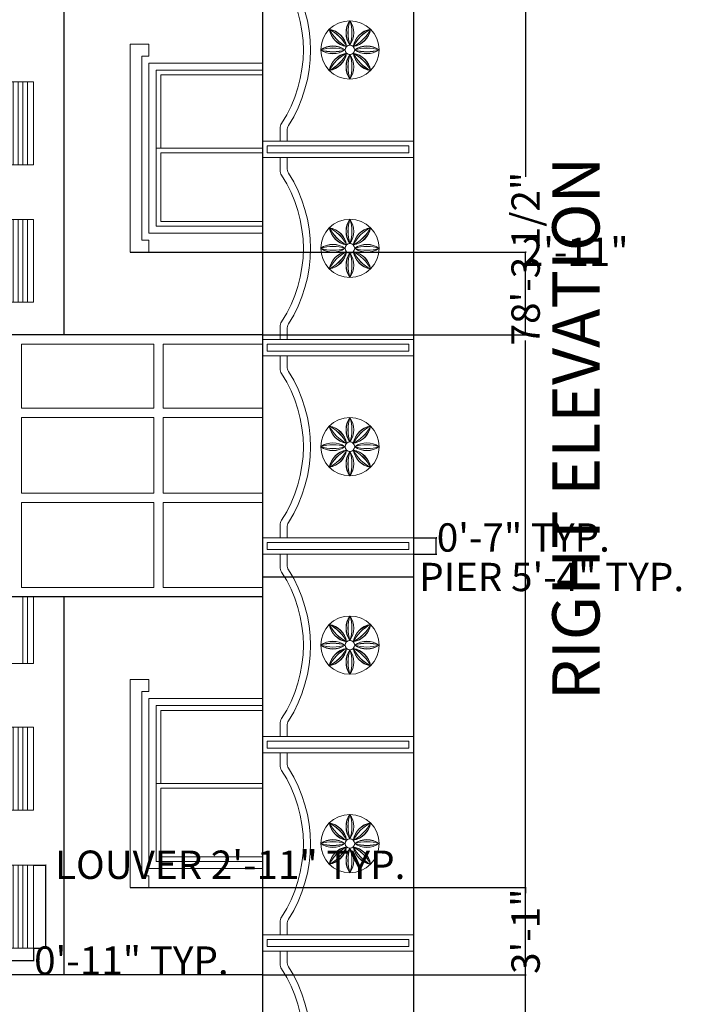
# Model space of a CAD drawing. Units: inches. Extents: x 1146 to 2917, y 889 to 2437.
# Tile 12 of 13: x 2585 to 2865, y 1586 to 2003. Entities that reach past the tile are written whole.
import ezdxf

# ---------------------------------------------------------------- set-up
doc = ezdxf.new("R2010")
doc.units = ezdxf.units.IN
doc.header["$MEASUREMENT"] = 0
for name, color, linetype, lineweight in [('A-ANNO-DIMS', 2, 'Continuous', 18), ('A-ANNO-TEXT', 7, 'Continuous', 25), ('A-ELEV', 7, 'Continuous', 30), ('A-ELEV-GLAZ', 5, 'Continuous', 18), ('A-ELEV-ORNM', 8, 'Continuous', 18)]:
    doc.layers.add(name, color=color, linetype=linetype, lineweight=lineweight)
doc.styles.get("Standard").update_dxf_attribs({"font": 'arial.ttf'})
doc.dimstyles.get("Standard").update_dxf_attribs({"dimtxt": 12, "dimasz": 0.18, "dimexe": 0.18, "dimexo": 0.0625, "dimgap": 0.09, "dimtad": 0, "dimtoh": 1, "dimdec": 1, "dimzin": 0, "dimdsep": 46, "dimlunit": 4, "dimtxsty": 'Standard', "dimcen": 0.09, "dimadec": 0, "dimazin": 0, "dimtfac": 1, "dimtdec": 1, "dimtofl": 0, "dimtmove": 0, "dimatfit": 3, "dimfxl": 1, "dimtolj": 1, "dimtzin": 0, "dimarcsym": 0})

# ---------------------------------------------------------------- blocks, each defined once
blk = doc.blocks.new('BOUNDARY-WALL-PIER')
for points in [[(0, 6.94), (64, 6.94), (64, 0), (0, 0)], [(2, 4.94), (62, 4.94), (62, 2), (2, 2)]]:
    blk.add_lwpolyline(points, close=True)
blk = doc.blocks.new('PARAPET-LOUVER')
for p, q in [((2.58, 0), (2.58, 35.13)), ((4.58, 0), (4.58, 35.13)), ((6.58, 0), (6.58, 35.13)), ((8.58, 0), (8.58, 35.13))]:
    blk.add_line(p, q)
blk.add_lwpolyline([(0, 0), (11.07, 0), (11.07, 35.13), (0, 35.13)], close=True)
blk = doc.blocks.new('WINDOW-ELEV-72')
for p, q in [((8, 83), (8, 88)), ((11, 44), (11, 77)), ((11, 77), (56, 77)), ((11, 11), (11, 44)), ((56, 44), (11, 44)), ((56, 11), (11, 11)), ((7.96, 5), (7.96, 0))]:
    blk.add_line(p, q)
for points in [[(7.96, 0), (0, 0), (0, 88), (8, 88)], [(7.96, 5), (5, 5), (5, 83), (8, 83)], [(56, 8), (8, 8), (8, 80), (56, 80)], [(13, 44), (13, 75), (56, 75)], [(13, 42), (56, 42)], [(56, 13), (13, 13), (13, 42)]]:
    blk.add_lwpolyline(points)
blk = doc.blocks.new('BOUNDARY-WALL-ARCH-CAP')
for p, q in [((0, 71.74), (0, 77.06)), ((3, 72.62), (3, 77.06)), ((0, 0), (0, 5.32)), ((3, 0), (3, 4.44))]:
    blk.add_line(p, q)
for centre, radius, start, end in [((4, 71.74), 4, 180, 213.079), ((7, 72.62), 4, 180, 212.2708), ((-46.98, 38.53), 56.85, 326.921, 33.079), ((-46.98, 38.53), 59.85, 327.7292, 32.2708), ((4, 5.32), 4, 146.921, 180), ((7, 4.44), 4, 147.7292, 180)]:
    blk.add_arc(centre, radius, start, end)
blk = doc.blocks.new('ROSETTE-PLANAR-TRACERY')
for radius in [12.33, 2.02]:
    blk.add_circle((12.33, 12.33), radius)
for centre, radius, start, end in [((2.21, 12.37), 8.8, 9.1552, 80.8448), ((12.65, 22.8), 9.21, 190.95, 259.05), ((19.96, 19.51), 9.21, 145.95, 214.05), ((5.2, 19.51), 8.8, 324.1552, 35.8448), ((12.37, 22.46), 8.8, 279.1552, 350.8448), ((22.8, 12.02), 9.21, 100.95, 169.05), ((5.15, 5.2), 8.8, 54.1552, 125.8448), ((19.51, 4.71), 9.21, 55.95, 124.05), ((5.15, 19.96), 9.21, 235.95, 304.05), ((12.3, 2.21), 8.8, 99.1552, 170.8448), ((1.86, 12.65), 9.21, 280.95, 349.05), ((19.47, 5.15), 8.8, 144.1552, 215.8448), ((4.71, 5.15), 9.21, 325.95, 34.05), ((22.46, 12.3), 8.8, 189.1552, 260.8448), ((12.02, 1.86), 9.21, 10.95, 79.05), ((19.51, 19.47), 8.8, 234.1552, 305.8448)]:
    blk.add_arc(centre, radius, start, end)
at = {"extrusion": (-2e-16, -2e-16, -1)}
for centre, radius, start, end in [((-12.3, 22.46), 8.8, 279.1552, 350.8448), ((-1.86, 12.02), 9.21, 100.95, 169.05)]:
    blk.add_arc(centre, radius, start, end, dxfattribs=at)
at = {"extrusion": (-2e-16, 0, -1)}
for centre, radius, start, end in [((-19.47, 19.51), 8.8, 324.1552, 35.8448), ((-4.71, 19.51), 9.21, 145.95, 214.05)]:
    blk.add_arc(centre, radius, start, end, dxfattribs=at)
at = {"extrusion": (-2e-16, 2e-16, -1)}
for centre, radius, start, end in [((-22.46, 12.37), 8.8, 9.1552, 80.8448), ((-12.02, 22.8), 9.21, 190.95, 259.05)]:
    blk.add_arc(centre, radius, start, end, dxfattribs=at)
at = {"extrusion": (0, -2e-16, -1)}
for centre, radius, start, end in [((-5.15, 4.71), 9.21, 55.95, 124.05), ((-5.15, 19.47), 8.8, 234.1552, 305.8448)]:
    blk.add_arc(centre, radius, start, end, dxfattribs=at)
at = {"extrusion": (0, 2e-16, -1)}
for centre, radius, start, end in [((-19.51, 5.2), 8.8, 54.1552, 125.8448), ((-19.51, 19.96), 9.21, 235.95, 304.05)]:
    blk.add_arc(centre, radius, start, end, dxfattribs=at)
at = {"extrusion": (2e-16, -2e-16, -1)}
for centre, radius, start, end in [((-2.21, 12.3), 8.8, 189.1552, 260.8448), ((-12.65, 1.86), 9.21, 10.95, 79.05)]:
    blk.add_arc(centre, radius, start, end, dxfattribs=at)
at = {"extrusion": (2e-16, 0, -1)}
for centre, radius, start, end in [((-19.96, 5.15), 9.21, 325.95, 34.05), ((-5.2, 5.15), 8.8, 144.1552, 215.8448)]:
    blk.add_arc(centre, radius, start, end, dxfattribs=at)
at = {"extrusion": (2e-16, 2e-16, -1)}
for centre, radius, start, end in [((-12.37, 2.21), 8.8, 99.1552, 170.8448), ((-22.8, 12.65), 9.21, 280.95, 349.05)]:
    blk.add_arc(centre, radius, start, end, dxfattribs=at)
blk = doc.blocks.new('*D83')
at = {"layer": 'A-ANNO-DIMS', "color": 0, "lineweight": -2, "transparency": 16777216}
for p, q in [((2688.2, 1776.39), (2688.2, 1766.67)), ((2752.2, 1776.39), (2752.2, 1766.67)), ((2688.38, 1766.85), (2752.02, 1766.85)), ((2752.2, 1766.85), (2752.38, 1766.85))]:
    blk.add_line(p, q, dxfattribs=at)
at = {"layer": 'A-ANNO-DIMS', "color": 0, "transparency": 16777216}
for points in [[(2688.38, 1766.88), (2688.38, 1766.82), (2688.2, 1766.85)], [(2752.02, 1766.88), (2752.02, 1766.82), (2752.2, 1766.85)]]:
    blk.add_solid(points, dxfattribs=at)
at = {"layer": 'Defpoints', "color": 0, "transparency": 16777216}
for p in [(2688.2, 1776.45), (2752.2, 1776.45), (2752.2, 1766.85)]:
    blk.add_point(p, dxfattribs=at)
at = {"layer": 'A-ANNO-DIMS', "color": 0, "transparency": 16777216, "insert": (2810.64, 1766.85), "char_height": 12, "attachment_point": 5}
blk.add_mtext('\\A1;PIER 5\'-4" TYP.', dxfattribs=at)
blk = doc.blocks.new('*D84')
at = {"layer": 'A-ANNO-DIMS', "color": 0, "lineweight": -2, "transparency": 16777216}
for p, q in [((2752.26, 1783.39), (2761.98, 1783.39)), ((2761.8, 1783.39), (2761.8, 1783.57)), ((2761.8, 1783.57), (2761.98, 1783.57)), ((2761.8, 1776.63), (2761.8, 1783.21)), ((2752.26, 1776.45), (2761.98, 1776.45))]:
    blk.add_line(p, q, dxfattribs=at)
at = {"layer": 'A-ANNO-DIMS', "color": 0, "transparency": 16777216}
for points in [[(2761.77, 1783.21), (2761.83, 1783.21), (2761.8, 1783.39)], [(2761.77, 1776.63), (2761.83, 1776.63), (2761.8, 1776.45)]]:
    blk.add_solid(points, dxfattribs=at)
at = {"layer": 'Defpoints', "color": 0, "transparency": 16777216}
for p in [(2752.2, 1783.39), (2761.8, 1783.39), (2752.2, 1776.45)]:
    blk.add_point(p, dxfattribs=at)
at = {"layer": 'A-ANNO-DIMS', "color": 0, "transparency": 16777216, "insert": (2798.64, 1783.57), "char_height": 12, "attachment_point": 5}
blk.add_mtext('\\A1;0\'-7" TYP.', dxfattribs=at)
blk = doc.blocks.new('*D89')
at = {"layer": 'A-ANNO-DIMS', "color": 0, "lineweight": -2, "transparency": 16777216}
for p, q in [((2591.33, 1644.85), (2596.72, 1644.85)), ((2596.54, 1644.85), (2596.54, 1645.03)), ((2596.54, 1645.03), (2596.72, 1645.03)), ((2596.54, 1609.9), (2596.54, 1644.67)), ((2591.33, 1609.72), (2596.72, 1609.72))]:
    blk.add_line(p, q, dxfattribs=at)
at = {"layer": 'A-ANNO-DIMS', "color": 0, "transparency": 16777216}
for points in [[(2596.51, 1644.67), (2596.57, 1644.67), (2596.54, 1644.85)], [(2596.51, 1609.9), (2596.57, 1609.9), (2596.54, 1609.72)]]:
    blk.add_solid(points, dxfattribs=at)
at = {"layer": 'Defpoints', "color": 0, "transparency": 16777216}
for p in [(2591.27, 1644.85), (2596.54, 1644.85), (2591.27, 1609.72)]:
    blk.add_point(p, dxfattribs=at)
at = {"layer": 'A-ANNO-DIMS', "color": 0, "transparency": 16777216, "insert": (2674.58, 1645.03), "char_height": 12, "attachment_point": 5}
blk.add_mtext('\\A1;LOUVER 2\'-11" TYP.', dxfattribs=at)
blk = doc.blocks.new('*D90')
at = {"layer": 'A-ANNO-DIMS', "color": 0, "lineweight": -2, "transparency": 16777216}
for p, q in [((2580.2, 1609.65), (2580.2, 1604.27)), ((2591.27, 1609.65), (2591.27, 1604.27)), ((2580.38, 1604.45), (2591.09, 1604.45)), ((2591.27, 1604.45), (2591.45, 1604.45))]:
    blk.add_line(p, q, dxfattribs=at)
at = {"layer": 'A-ANNO-DIMS', "color": 0, "transparency": 16777216}
for points in [[(2580.38, 1604.48), (2580.38, 1604.42), (2580.2, 1604.45)], [(2591.09, 1604.48), (2591.09, 1604.42), (2591.27, 1604.45)]]:
    blk.add_solid(points, dxfattribs=at)
at = {"layer": 'Defpoints', "color": 0, "transparency": 16777216}
for p in [(2580.2, 1609.72), (2591.27, 1609.72), (2591.27, 1604.45)]:
    blk.add_point(p, dxfattribs=at)
at = {"layer": 'A-ANNO-DIMS', "color": 0, "transparency": 16777216, "insert": (2632.77, 1604.45), "char_height": 12, "attachment_point": 5}
blk.add_mtext('\\A1;0\'-11" TYP.', dxfattribs=at)
blk = doc.blocks.new('*D121')
at = {"layer": 'A-ANNO-DIMS', "color": 0, "lineweight": -2, "transparency": 16777216}
for p, q in [((2752.26, 2371.39), (2799.78, 2371.39)), ((2799.6, 2371.21), (2799.6, 1936.27)), ((2799.6, 1432.07), (2799.6, 1867.01)), ((2752.26, 1431.89), (2799.78, 1431.89))]:
    blk.add_line(p, q, dxfattribs=at)
at = {"layer": 'A-ANNO-DIMS', "color": 0, "transparency": 16777216}
for points in [[(2799.57, 2371.21), (2799.63, 2371.21), (2799.6, 2371.39)], [(2799.57, 1432.07), (2799.63, 1432.07), (2799.6, 1431.89)]]:
    blk.add_solid(points, dxfattribs=at)
at = {"layer": 'Defpoints', "color": 0, "transparency": 16777216}
for p in [(2752.2, 2371.39), (2799.6, 2371.39), (2752.2, 1431.89)]:
    blk.add_point(p, dxfattribs=at)
at = {"layer": 'A-ANNO-DIMS', "color": 0, "transparency": 16777216, "insert": (2799.6, 1901.64), "char_height": 12, "attachment_point": 5, "rotation": 90}
blk.add_mtext('\\A1;78\'-3 1/2"', dxfattribs=at)
blk = doc.blocks.new('*D122')
at = {"layer": 'A-ANNO-DIMS', "color": 0, "lineweight": -2, "transparency": 16777216}
for p, q in [((2460.2, 1869.45), (2460.2, 2418.97)), ((2460.38, 2418.79), (2585.4, 2418.79)), ((2752.02, 2418.79), (2627, 2418.79)), ((2752.2, 2371.45), (2752.2, 2418.97))]:
    blk.add_line(p, q, dxfattribs=at)
at = {"layer": 'A-ANNO-DIMS', "color": 0, "transparency": 16777216}
for points in [[(2460.38, 2418.82), (2460.38, 2418.76), (2460.2, 2418.79)], [(2752.02, 2418.82), (2752.02, 2418.76), (2752.2, 2418.79)]]:
    blk.add_solid(points, dxfattribs=at)
at = {"layer": 'Defpoints', "color": 0, "transparency": 16777216}
for p in [(2752.2, 2418.79), (2752.2, 2371.39), (2460.2, 1869.39)]:
    blk.add_point(p, dxfattribs=at)
at = {"layer": 'A-ANNO-DIMS', "color": 0, "transparency": 16777216, "insert": (2606.2, 2418.79), "char_height": 12, "attachment_point": 5}
blk.add_mtext('\\A1;24\'-4"', dxfattribs=at)
blk = doc.blocks.new('*D128')
at = {"layer": 'A-ANNO-DIMS', "color": 0, "lineweight": -2, "transparency": 16777216}
for p, q in [((2580.2, 1598.33), (2580.2, 1384.31)), ((2752.2, 1431.83), (2752.2, 1384.31)), ((2580.38, 1384.49), (2646.06, 1384.49)), ((2752.02, 1384.49), (2686.34, 1384.49))]:
    blk.add_line(p, q, dxfattribs=at)
at = {"layer": 'A-ANNO-DIMS', "color": 0, "transparency": 16777216}
for points in [[(2580.38, 1384.52), (2580.38, 1384.46), (2580.2, 1384.49)], [(2752.02, 1384.52), (2752.02, 1384.46), (2752.2, 1384.49)]]:
    blk.add_solid(points, dxfattribs=at)
at = {"layer": 'Defpoints', "color": 0, "transparency": 16777216}
for p in [(2580.2, 1598.39), (2752.2, 1431.89), (2752.2, 1384.49)]:
    blk.add_point(p, dxfattribs=at)
at = {"layer": 'A-ANNO-DIMS', "color": 0, "transparency": 16777216, "insert": (2666.2, 1384.49), "char_height": 12, "attachment_point": 5}
blk.add_mtext('\\A1;14\'-4"', dxfattribs=at)
blk = doc.blocks.new('*D129')
at = {"layer": 'A-ANNO-DIMS', "color": 0, "lineweight": -2, "transparency": 16777216}
for p, q in [((2580.14, 1598.39), (2412.62, 1598.39)), ((2412.8, 1598.21), (2412.8, 1553.92)), ((2412.8, 1432.07), (2412.8, 1476.36)), ((2752.14, 1431.89), (2412.62, 1431.89))]:
    blk.add_line(p, q, dxfattribs=at)
at = {"layer": 'A-ANNO-DIMS', "color": 0, "transparency": 16777216}
for points in [[(2412.77, 1598.21), (2412.83, 1598.21), (2412.8, 1598.39)], [(2412.77, 1432.07), (2412.83, 1432.07), (2412.8, 1431.89)]]:
    blk.add_solid(points, dxfattribs=at)
at = {"layer": 'Defpoints', "color": 0, "transparency": 16777216}
for p in [(2580.2, 1598.39), (2412.8, 1431.89), (2752.2, 1431.89)]:
    blk.add_point(p, dxfattribs=at)
at = {"layer": 'A-ANNO-DIMS', "color": 0, "transparency": 16777216, "insert": (2412.8, 1515.14), "char_height": 12, "attachment_point": 5, "rotation": 90}
blk.add_mtext('\\A1;13\'-10 1/2"', dxfattribs=at)
blk = doc.blocks.new('*D138')
at = {"layer": 'A-ANNO-DIMS', "color": 0, "lineweight": -2, "transparency": 16777216}
for p, q in [((2632.26, 1635.39), (2799.78, 1635.39)), ((2799.6, 1635.21), (2799.6, 1632.93)), ((2799.6, 1598.57), (2799.6, 1600.86)), ((2688.26, 1598.39), (2799.78, 1598.39))]:
    blk.add_line(p, q, dxfattribs=at)
at = {"layer": 'A-ANNO-DIMS', "color": 0, "transparency": 16777216}
for points in [[(2799.57, 1635.21), (2799.63, 1635.21), (2799.6, 1635.39)], [(2799.57, 1598.57), (2799.63, 1598.57), (2799.6, 1598.39)]]:
    blk.add_solid(points, dxfattribs=at)
at = {"layer": 'Defpoints', "color": 0, "transparency": 16777216}
for p in [(2632.2, 1635.39), (2799.6, 1635.39), (2688.2, 1598.39)]:
    blk.add_point(p, dxfattribs=at)
at = {"layer": 'A-ANNO-DIMS', "color": 0, "transparency": 16777216, "insert": (2799.6, 1616.89), "char_height": 12, "attachment_point": 5, "rotation": 90}
blk.add_mtext('\\A1;3\'-1"', dxfattribs=at)
blk = doc.blocks.new('*D139')
at = {"layer": 'A-ANNO-DIMS', "color": 0, "lineweight": -2, "transparency": 16777216}
for p, q in [((2632.26, 1904.39), (2799.78, 1904.39)), ((2799.6, 1904.39), (2799.6, 1904.57)), ((2799.6, 1904.57), (2799.78, 1904.57)), ((2799.6, 1869.57), (2799.6, 1904.21)), ((2688.26, 1869.39), (2799.78, 1869.39))]:
    blk.add_line(p, q, dxfattribs=at)
at = {"layer": 'A-ANNO-DIMS', "color": 0, "transparency": 16777216}
for points in [[(2799.57, 1904.21), (2799.63, 1904.21), (2799.6, 1904.39)], [(2799.57, 1869.57), (2799.63, 1869.57), (2799.6, 1869.39)]]:
    blk.add_solid(points, dxfattribs=at)
at = {"layer": 'Defpoints', "color": 0, "transparency": 16777216}
for p in [(2632.2, 1904.39), (2799.6, 1904.39), (2688.2, 1869.39)]:
    blk.add_point(p, dxfattribs=at)
at = {"layer": 'A-ANNO-DIMS', "color": 0, "transparency": 16777216, "insert": (2820.58, 1904.57), "char_height": 12, "attachment_point": 5}
blk.add_mtext('\\A1;2\'-11"', dxfattribs=at)

msp = doc.modelspace()

# ---------------------------------------------------------------- linework, layer by layer
at = {"layer": 'A-ELEV'}
for p, q in [((2752.2, 2371.39), (2752.2, 1431.89)), ((2604.2, 2182.39), (2604.2, 1869.39)), ((2688.2, 2182.39), (2688.2, 1431.89)), ((2688.2, 1869.39), (2460.2, 1869.39)), ((2688.2, 1758.39), (2460.2, 1758.39)), ((2604.2, 1758.39), (2604.2, 1598.39)), ((2688.2, 1598.39), (2580.2, 1598.39))]:
    msp.add_line(p, q, dxfattribs=at)
at = {"layer": 'A-ELEV-GLAZ'}
for p, q in [((2640.2, 1987.39), (2640.2, 1992.39)), ((2643.2, 1948.39), (2643.2, 1981.39)), ((2643.2, 1981.39), (2688.2, 1981.39)), ((2643.2, 1948.39), (2643.2, 1981.39)), ((2643.2, 1981.39), (2688.2, 1981.39)), ((2643.2, 1915.39), (2643.2, 1948.39)), ((2643.2, 1915.39), (2643.2, 1948.39)), ((2688.2, 1948.39), (2643.2, 1948.39)), ((2688.2, 1948.39), (2643.2, 1948.39)), ((2688.2, 1915.39), (2643.2, 1915.39)), ((2688.2, 1915.39), (2643.2, 1915.39)), ((2640.16, 1909.39), (2640.16, 1904.39)), ((2586.2, 1865.39), (2586.2, 1838.39)), ((2642.2, 1865.39), (2586.2, 1865.39)), ((2642.2, 1865.39), (2642.2, 1838.39)), ((2646.2, 1865.39), (2646.2, 1838.39)), ((2688.2, 1865.39), (2646.2, 1865.39)), ((2642.2, 1838.39), (2586.2, 1838.39)), ((2688.2, 1838.39), (2646.2, 1838.39)), ((2586.2, 1834.39), (2586.2, 1802.39)), ((2642.2, 1834.39), (2586.2, 1834.39)), ((2642.2, 1834.39), (2642.2, 1802.39)), ((2688.2, 1834.39), (2646.2, 1834.39)), ((2646.2, 1834.39), (2646.2, 1802.39)), ((2642.2, 1802.39), (2586.2, 1802.39)), ((2688.2, 1802.39), (2646.2, 1802.39)), ((2586.2, 1798.39), (2586.2, 1762.39)), ((2642.2, 1798.39), (2586.2, 1798.39)), ((2642.2, 1798.39), (2642.2, 1762.39)), ((2688.2, 1798.39), (2646.2, 1798.39)), ((2646.2, 1798.39), (2646.2, 1762.39)), ((2642.2, 1762.39), (2586.2, 1762.39)), ((2688.2, 1762.39), (2646.2, 1762.39))]:
    msp.add_line(p, q, dxfattribs=at)
for points in [[(2640.16, 1904.39), (2632.2, 1904.39), (2632.2, 1992.39), (2640.2, 1992.39)], [(2640.16, 1909.39), (2637.2, 1909.39), (2637.2, 1987.39), (2640.2, 1987.39)], [(2688.2, 1912.39), (2640.2, 1912.39), (2640.2, 1984.39), (2688.2, 1984.39)], [(2688.2, 1912.39), (2640.2, 1912.39), (2640.2, 1984.39), (2688.2, 1984.39)], [(2645.2, 1948.39), (2645.2, 1979.39), (2688.2, 1979.39)], [(2645.2, 1948.39), (2645.2, 1979.39), (2688.2, 1979.39)], [(2645.2, 1946.39), (2688.2, 1946.39)], [(2645.2, 1946.39), (2688.2, 1946.39)], [(2688.2, 1917.39), (2645.2, 1917.39), (2645.2, 1946.39)], [(2688.2, 1917.39), (2645.2, 1917.39), (2645.2, 1946.39)]]:
    msp.add_lwpolyline(points, dxfattribs=at)
at = {"layer": 'A-ELEV-ORNM'}
for p, q in [((2586.78, 1730.24), (2586.78, 1758.39)), ((2588.78, 1730.24), (2588.78, 1758.39))]:
    msp.add_line(p, q, dxfattribs=at)
msp.add_lwpolyline([(2580.2, 1758.39), (2580.2, 1730.24), (2591.27, 1730.24), (2591.27, 1758.39)], dxfattribs=at)
at = {"layer": 'A-ELEV-ORNM', "extrusion": (0.866025, 5.48447e-11, -0.5)}
for centre, radius, start, end in [((1997.18, 1369.76, 2360.14), 8.8, 234.1552, 305.8448), ((1997.18, 1355, 2360.14), 9.21, 55.95, 124.05), ((1913.18, 1369.76, 2360.14), 8.8, 234.1552, 305.8448), ((1913.18, 1355, 2360.14), 9.21, 55.95, 124.05), ((1829.18, 1369.76, 2360.14), 8.8, 234.1552, 305.8448), ((1829.18, 1355, 2360.14), 9.21, 55.95, 124.05), ((1745.18, 1369.76, 2360.14), 8.8, 234.1552, 305.8448), ((1745.18, 1355, 2360.14), 9.21, 55.95, 124.05), ((1661.18, 1369.76, 2360.14), 8.8, 234.1552, 305.8448), ((1661.18, 1355, 2360.14), 9.21, 55.95, 124.05)]:
    msp.add_arc(centre, radius, start, end, dxfattribs=at)
at = {"layer": 'A-ELEV-ORNM', "extrusion": (-0.866025, -5.48447e-11, -0.5)}
for centre, radius, start, end in [((-1997.18, -1369.76, -2360.14), 8.8, 54.1552, 125.8448), ((-1997.18, -1355, -2360.14), 9.21, 235.95, 304.05), ((-1913.18, -1369.76, -2360.14), 8.8, 54.1552, 125.8448), ((-1913.18, -1355, -2360.14), 9.21, 235.95, 304.05), ((-1829.18, -1369.76, -2360.14), 8.8, 54.1552, 125.8448), ((-1829.18, -1355, -2360.14), 9.21, 235.95, 304.05), ((-1745.18, -1369.76, -2360.14), 8.8, 54.1552, 125.8448), ((-1745.18, -1355, -2360.14), 9.21, 235.95, 304.05), ((-1661.18, -1369.76, -2360.14), 8.8, 54.1552, 125.8448), ((-1661.18, -1355, -2360.14), 9.21, 235.95, 304.05)]:
    msp.add_arc(centre, radius, start, end, dxfattribs=at)
at = {"layer": 'A-ELEV-ORNM', "extrusion": (0.866025, 5.48447e-11, 0.5)}
for centre, radius, start, end in [((1997.18, -1370.26, 2360.14), 9.21, 55.95, 124.05), ((1997.18, -1355.49, 2360.14), 8.8, 234.1552, 305.8448), ((1913.18, -1370.26, 2360.14), 9.21, 55.95, 124.05), ((1913.18, -1355.49, 2360.14), 8.8, 234.1552, 305.8448), ((1829.18, -1370.26, 2360.14), 9.21, 55.95, 124.05), ((1829.18, -1355.49, 2360.14), 8.8, 234.1552, 305.8448), ((1745.18, -1370.26, 2360.14), 9.21, 55.95, 124.05), ((1745.18, -1355.49, 2360.14), 8.8, 234.1552, 305.8448), ((1661.18, -1370.26, 2360.14), 9.21, 55.95, 124.05), ((1661.18, -1355.49, 2360.14), 8.8, 234.1552, 305.8448)]:
    msp.add_arc(centre, radius, start, end, dxfattribs=at)
at = {"layer": 'A-ELEV-ORNM', "extrusion": (-0.866025, -5.48447e-11, 0.5)}
for centre, radius, start, end in [((-1997.18, 1370.26, -2360.14), 9.21, 235.95, 304.05), ((-1997.18, 1355.49, -2360.14), 8.8, 54.1552, 125.8448), ((-1913.18, 1370.26, -2360.14), 9.21, 235.95, 304.05), ((-1913.18, 1355.49, -2360.14), 8.8, 54.1552, 125.8448), ((-1829.18, 1370.26, -2360.14), 9.21, 235.95, 304.05), ((-1829.18, 1355.49, -2360.14), 8.8, 54.1552, 125.8448), ((-1745.18, 1370.26, -2360.14), 9.21, 235.95, 304.05), ((-1745.18, 1355.49, -2360.14), 8.8, 54.1552, 125.8448), ((-1661.18, 1370.26, -2360.14), 9.21, 235.95, 304.05), ((-1661.18, 1355.49, -2360.14), 8.8, 54.1552, 125.8448)]:
    msp.add_arc(centre, radius, start, end, dxfattribs=at)
at = {"layer": 'A-ELEV-ORNM', "extrusion": (0.612372, 0.612372, 0.5)}
for centre, radius, start, end in [((-512.72, -1659.96, 2887.49), 8.8, 234.1552, 305.8448), ((-512.72, -1674.72, 2887.49), 9.21, 55.95, 124.05), ((-527.08, -1674.23, 2887.49), 8.8, 54.1552, 125.8448), ((-527.08, -1659.47, 2887.49), 9.21, 235.95, 304.05), ((-572.12, -1630.26, 2836.06), 8.8, 234.1552, 305.8448), ((-572.12, -1645.02, 2836.06), 9.21, 55.95, 124.05), ((-586.48, -1644.53, 2836.06), 8.8, 54.1552, 125.8448), ((-586.48, -1629.77, 2836.06), 9.21, 235.95, 304.05), ((-631.52, -1600.56, 2784.62), 8.8, 234.1552, 305.8448), ((-631.52, -1615.33, 2784.62), 9.21, 55.95, 124.05), ((-645.88, -1614.83, 2784.62), 8.8, 54.1552, 125.8448), ((-645.88, -1600.07, 2784.62), 9.21, 235.95, 304.05), ((-690.91, -1570.87, 2733.18), 8.8, 234.1552, 305.8448), ((-690.91, -1585.63, 2733.18), 9.21, 55.95, 124.05), ((-705.27, -1585.14, 2733.18), 8.8, 54.1552, 125.8448), ((-705.27, -1570.37, 2733.18), 9.21, 235.95, 304.05), ((-750.31, -1541.17, 2681.74), 8.8, 234.1552, 305.8448), ((-750.31, -1555.93, 2681.74), 9.21, 55.95, 124.05), ((-764.67, -1555.44, 2681.74), 8.8, 54.1552, 125.8448), ((-764.67, -1540.67, 2681.74), 9.21, 235.95, 304.05)]:
    msp.add_arc(centre, radius, start, end, dxfattribs=at)
at = {"layer": 'A-ELEV-ORNM', "extrusion": (0.612372, 0.612372, -0.5)}
for centre, radius, start, end in [((-512.72, 1674.23, 2887.49), 8.8, 234.1552, 305.8448), ((-512.72, 1659.47, 2887.49), 9.21, 55.95, 124.05), ((-527.08, 1659.96, 2887.49), 8.8, 54.1552, 125.8448), ((-527.08, 1674.72, 2887.49), 9.21, 235.95, 304.05), ((-572.12, 1644.53, 2836.06), 8.8, 234.1552, 305.8448), ((-572.12, 1629.77, 2836.06), 9.21, 55.95, 124.05), ((-586.48, 1630.26, 2836.06), 8.8, 54.1552, 125.8448), ((-586.48, 1645.02, 2836.06), 9.21, 235.95, 304.05), ((-631.52, 1614.83, 2784.62), 8.8, 234.1552, 305.8448), ((-631.52, 1600.07, 2784.62), 9.21, 55.95, 124.05), ((-645.88, 1600.56, 2784.62), 8.8, 54.1552, 125.8448), ((-645.88, 1615.33, 2784.62), 9.21, 235.95, 304.05), ((-690.91, 1585.14, 2733.18), 8.8, 234.1552, 305.8448), ((-690.91, 1570.37, 2733.18), 9.21, 55.95, 124.05), ((-705.27, 1570.87, 2733.18), 8.8, 54.1552, 125.8448), ((-705.27, 1585.63, 2733.18), 9.21, 235.95, 304.05), ((-750.31, 1555.44, 2681.74), 8.8, 234.1552, 305.8448), ((-750.31, 1540.67, 2681.74), 9.21, 55.95, 124.05), ((-764.67, 1541.17, 2681.74), 8.8, 54.1552, 125.8448), ((-764.67, 1555.93, 2681.74), 9.21, 235.95, 304.05)]:
    msp.add_arc(centre, radius, start, end, dxfattribs=at)
at = {"layer": 'A-ELEV-ORNM', "extrusion": (-0.612372, -0.612372, -0.5)}
for centre, radius, start, end in [((512.72, -1674.23, -2887.49), 8.8, 54.1552, 125.8448), ((512.72, -1659.47, -2887.49), 9.21, 235.95, 304.05), ((527.08, -1659.96, -2887.49), 8.8, 234.1552, 305.8448), ((527.08, -1674.72, -2887.49), 9.21, 55.95, 124.05), ((572.12, -1644.53, -2836.06), 8.8, 54.1552, 125.8448), ((572.12, -1629.77, -2836.06), 9.21, 235.95, 304.05), ((586.48, -1630.26, -2836.06), 8.8, 234.1552, 305.8448), ((586.48, -1645.02, -2836.06), 9.21, 55.95, 124.05), ((631.52, -1614.83, -2784.62), 8.8, 54.1552, 125.8448), ((631.52, -1600.07, -2784.62), 9.21, 235.95, 304.05), ((645.88, -1600.56, -2784.62), 8.8, 234.1552, 305.8448), ((645.88, -1615.33, -2784.62), 9.21, 55.95, 124.05), ((690.91, -1585.14, -2733.18), 8.8, 54.1552, 125.8448), ((690.91, -1570.37, -2733.18), 9.21, 235.95, 304.05), ((705.27, -1570.87, -2733.18), 8.8, 234.1552, 305.8448), ((705.27, -1585.63, -2733.18), 9.21, 55.95, 124.05), ((750.31, -1555.44, -2681.74), 8.8, 54.1552, 125.8448), ((750.31, -1540.67, -2681.74), 9.21, 235.95, 304.05), ((764.67, -1541.17, -2681.74), 8.8, 234.1552, 305.8448), ((764.67, -1555.93, -2681.74), 9.21, 55.95, 124.05)]:
    msp.add_arc(centre, radius, start, end, dxfattribs=at)
at = {"layer": 'A-ELEV-ORNM', "extrusion": (-0.612372, -0.612372, 0.5)}
for centre, radius, start, end in [((512.72, 1659.96, -2887.49), 8.8, 54.1552, 125.8448), ((512.72, 1674.72, -2887.49), 9.21, 235.95, 304.05), ((527.08, 1674.23, -2887.49), 8.8, 234.1552, 305.8448), ((527.08, 1659.47, -2887.49), 9.21, 55.95, 124.05), ((572.12, 1630.26, -2836.06), 8.8, 54.1552, 125.8448), ((572.12, 1645.02, -2836.06), 9.21, 235.95, 304.05), ((586.48, 1644.53, -2836.06), 8.8, 234.1552, 305.8448), ((586.48, 1629.77, -2836.06), 9.21, 55.95, 124.05), ((631.52, 1600.56, -2784.62), 8.8, 54.1552, 125.8448), ((631.52, 1615.33, -2784.62), 9.21, 235.95, 304.05), ((645.88, 1614.83, -2784.62), 8.8, 234.1552, 305.8448), ((645.88, 1600.07, -2784.62), 9.21, 55.95, 124.05), ((690.91, 1570.87, -2733.18), 8.8, 54.1552, 125.8448), ((690.91, 1585.63, -2733.18), 9.21, 235.95, 304.05), ((705.27, 1585.14, -2733.18), 8.8, 234.1552, 305.8448), ((705.27, 1570.37, -2733.18), 9.21, 55.95, 124.05), ((750.31, 1541.17, -2681.74), 8.8, 54.1552, 125.8448), ((750.31, 1555.93, -2681.74), 9.21, 235.95, 304.05), ((764.67, 1555.44, -2681.74), 8.8, 234.1552, 305.8448), ((764.67, 1540.67, -2681.74), 9.21, 55.95, 124.05)]:
    msp.add_arc(centre, radius, start, end, dxfattribs=at)
at = {"layer": 'A-ELEV-ORNM', "extrusion": (0.612372, -0.612372, 0.5)}
for centre, radius, start, end in [((3341.37, -252.82, 450.25), 8.8, 234.1552, 305.8448), ((3341.37, -267.58, 450.25), 9.21, 55.95, 124.05), ((3327.01, -267.09, 450.25), 8.8, 54.1552, 125.8448), ((3327.01, -252.32, 450.25), 9.21, 235.95, 304.05), ((3281.97, -282.51, 501.69), 8.8, 234.1552, 305.8448), ((3281.97, -297.28, 501.69), 9.21, 55.95, 124.05), ((3267.62, -296.78, 501.69), 8.8, 54.1552, 125.8448), ((3267.62, -282.02, 501.69), 9.21, 235.95, 304.05), ((3222.58, -312.21, 553.13), 8.8, 234.1552, 305.8448), ((3222.58, -326.98, 553.13), 9.21, 55.95, 124.05), ((3208.22, -326.48, 553.13), 8.8, 54.1552, 125.8448), ((3208.22, -311.72, 553.13), 9.21, 235.95, 304.05), ((3163.18, -341.91, 604.57), 8.8, 234.1552, 305.8448), ((3163.18, -356.67, 604.57), 9.21, 55.95, 124.05), ((3148.82, -356.18, 604.57), 8.8, 54.1552, 125.8448), ((3148.82, -341.42, 604.57), 9.21, 235.95, 304.05), ((3103.78, -371.61, 656.01), 8.8, 234.1552, 305.8448), ((3103.78, -386.37, 656.01), 9.21, 55.95, 124.05), ((3089.42, -385.88, 656.01), 8.8, 54.1552, 125.8448), ((3089.42, -371.12, 656.01), 9.21, 235.95, 304.05)]:
    msp.add_arc(centre, radius, start, end, dxfattribs=at)
at = {"layer": 'A-ELEV-ORNM', "extrusion": (0.612372, -0.612372, -0.5)}
for centre, radius, start, end in [((3341.37, 267.09, 450.25), 8.8, 234.1552, 305.8448), ((3341.37, 252.32, 450.25), 9.21, 55.95, 124.05), ((3327.01, 252.82, 450.25), 8.8, 54.1552, 125.8448), ((3327.01, 267.58, 450.25), 9.21, 235.95, 304.05), ((3281.97, 296.78, 501.69), 8.8, 234.1552, 305.8448), ((3281.97, 282.02, 501.69), 9.21, 55.95, 124.05), ((3267.62, 282.51, 501.69), 8.8, 54.1552, 125.8448), ((3267.62, 297.28, 501.69), 9.21, 235.95, 304.05), ((3222.58, 326.48, 553.13), 8.8, 234.1552, 305.8448), ((3222.58, 311.72, 553.13), 9.21, 55.95, 124.05), ((3208.22, 312.21, 553.13), 8.8, 54.1552, 125.8448), ((3208.22, 326.98, 553.13), 9.21, 235.95, 304.05), ((3163.18, 356.18, 604.57), 8.8, 234.1552, 305.8448), ((3163.18, 341.42, 604.57), 9.21, 55.95, 124.05), ((3148.82, 341.91, 604.57), 8.8, 54.1552, 125.8448), ((3148.82, 356.67, 604.57), 9.21, 235.95, 304.05), ((3103.78, 385.88, 656.01), 8.8, 234.1552, 305.8448), ((3103.78, 371.12, 656.01), 9.21, 55.95, 124.05), ((3089.42, 371.61, 656.01), 8.8, 54.1552, 125.8448), ((3089.42, 386.37, 656.01), 9.21, 235.95, 304.05)]:
    msp.add_arc(centre, radius, start, end, dxfattribs=at)
at = {"layer": 'A-ELEV-ORNM', "extrusion": (-0.612372, 0.612372, -0.5)}
for centre, radius, start, end in [((-3341.37, -267.09, -450.25), 8.8, 54.1552, 125.8448), ((-3341.37, -252.32, -450.25), 9.21, 235.95, 304.05), ((-3327.01, -252.82, -450.25), 8.8, 234.1552, 305.8448), ((-3327.01, -267.58, -450.25), 9.21, 55.95, 124.05), ((-3281.97, -296.78, -501.69), 8.8, 54.1552, 125.8448), ((-3281.97, -282.02, -501.69), 9.21, 235.95, 304.05), ((-3267.62, -282.51, -501.69), 8.8, 234.1552, 305.8448), ((-3267.62, -297.28, -501.69), 9.21, 55.95, 124.05), ((-3222.58, -326.48, -553.13), 8.8, 54.1552, 125.8448), ((-3222.58, -311.72, -553.13), 9.21, 235.95, 304.05), ((-3208.22, -312.21, -553.13), 8.8, 234.1552, 305.8448), ((-3208.22, -326.98, -553.13), 9.21, 55.95, 124.05), ((-3163.18, -356.18, -604.57), 8.8, 54.1552, 125.8448), ((-3163.18, -341.42, -604.57), 9.21, 235.95, 304.05), ((-3148.82, -341.91, -604.57), 8.8, 234.1552, 305.8448), ((-3148.82, -356.67, -604.57), 9.21, 55.95, 124.05), ((-3103.78, -385.88, -656.01), 8.8, 54.1552, 125.8448), ((-3103.78, -371.12, -656.01), 9.21, 235.95, 304.05), ((-3089.42, -371.61, -656.01), 8.8, 234.1552, 305.8448), ((-3089.42, -386.37, -656.01), 9.21, 55.95, 124.05)]:
    msp.add_arc(centre, radius, start, end, dxfattribs=at)
at = {"layer": 'A-ELEV-ORNM', "extrusion": (-0.612372, 0.612372, 0.5)}
for centre, radius, start, end in [((-3341.37, 252.82, -450.25), 8.8, 54.1552, 125.8448), ((-3341.37, 267.58, -450.25), 9.21, 235.95, 304.05), ((-3327.01, 267.09, -450.25), 8.8, 234.1552, 305.8448), ((-3327.01, 252.32, -450.25), 9.21, 55.95, 124.05), ((-3281.97, 282.51, -501.69), 8.8, 54.1552, 125.8448), ((-3281.97, 297.28, -501.69), 9.21, 235.95, 304.05), ((-3267.62, 296.78, -501.69), 8.8, 234.1552, 305.8448), ((-3267.62, 282.02, -501.69), 9.21, 55.95, 124.05), ((-3222.58, 312.21, -553.13), 8.8, 54.1552, 125.8448), ((-3222.58, 326.98, -553.13), 9.21, 235.95, 304.05), ((-3208.22, 326.48, -553.13), 8.8, 234.1552, 305.8448), ((-3208.22, 311.72, -553.13), 9.21, 55.95, 124.05), ((-3163.18, 341.91, -604.57), 8.8, 54.1552, 125.8448), ((-3163.18, 356.67, -604.57), 9.21, 235.95, 304.05), ((-3148.82, 356.18, -604.57), 8.8, 234.1552, 305.8448), ((-3148.82, 341.42, -604.57), 9.21, 55.95, 124.05), ((-3103.78, 371.61, -656.01), 8.8, 54.1552, 125.8448), ((-3103.78, 386.37, -656.01), 9.21, 235.95, 304.05), ((-3089.42, 385.88, -656.01), 8.8, 234.1552, 305.8448), ((-3089.42, 371.12, -656.01), 9.21, 55.95, 124.05)]:
    msp.add_arc(centre, radius, start, end, dxfattribs=at)
at = {"layer": 'A-ELEV-ORNM', "extrusion": (-5.48444e-11, 0.866025, 0.5)}
for centre, radius, start, end in [((-2718.08, -987.87, 1723.39), 8.8, 234.1552, 305.8448), ((-2718.08, -1002.63, 1723.39), 9.21, 55.95, 124.05), ((-2732.44, -987.37, 1723.39), 9.21, 235.95, 304.05), ((-2732.44, -1002.14, 1723.39), 8.8, 54.1552, 125.8448), ((-2718.08, -945.87, 1650.65), 8.8, 234.1552, 305.8448), ((-2718.08, -960.63, 1650.65), 9.21, 55.95, 124.05), ((-2732.44, -945.37, 1650.65), 9.21, 235.95, 304.05), ((-2732.44, -960.14, 1650.65), 8.8, 54.1552, 125.8448), ((-2718.08, -903.87, 1577.9), 8.8, 234.1552, 305.8448), ((-2718.08, -918.63, 1577.9), 9.21, 55.95, 124.05), ((-2732.44, -903.37, 1577.9), 9.21, 235.95, 304.05), ((-2732.44, -918.14, 1577.9), 8.8, 54.1552, 125.8448), ((-2718.08, -861.87, 1505.15), 8.8, 234.1552, 305.8448), ((-2732.44, -861.37, 1505.15), 9.21, 235.95, 304.05), ((-2718.08, -876.63, 1505.15), 9.21, 55.95, 124.05), ((-2732.44, -876.14, 1505.15), 8.8, 54.1552, 125.8448), ((-2718.08, -819.87, 1432.41), 8.8, 234.1552, 305.8448), ((-2732.44, -819.37, 1432.41), 9.21, 235.95, 304.05), ((-2718.08, -834.63, 1432.41), 9.21, 55.95, 124.05), ((-2732.44, -834.14, 1432.41), 8.8, 54.1552, 125.8448)]:
    msp.add_arc(centre, radius, start, end, dxfattribs=at)
at = {"layer": 'A-ELEV-ORNM', "extrusion": (5.48444e-11, -0.866025, 0.5)}
for centre, radius, start, end in [((2718.08, 987.87, -1723.39), 8.8, 54.1552, 125.8448), ((2718.08, 1002.63, -1723.39), 9.21, 235.95, 304.05), ((2732.44, 987.37, -1723.39), 9.21, 55.95, 124.05), ((2732.44, 1002.14, -1723.39), 8.8, 234.1552, 305.8448), ((2718.08, 945.87, -1650.65), 8.8, 54.1552, 125.8448), ((2718.08, 960.63, -1650.65), 9.21, 235.95, 304.05), ((2732.44, 945.37, -1650.65), 9.21, 55.95, 124.05), ((2732.44, 960.14, -1650.65), 8.8, 234.1552, 305.8448), ((2718.08, 903.87, -1577.9), 8.8, 54.1552, 125.8448), ((2718.08, 918.63, -1577.9), 9.21, 235.95, 304.05), ((2732.44, 903.37, -1577.9), 9.21, 55.95, 124.05), ((2732.44, 918.14, -1577.9), 8.8, 234.1552, 305.8448), ((2718.08, 861.87, -1505.15), 8.8, 54.1552, 125.8448), ((2732.44, 861.37, -1505.15), 9.21, 55.95, 124.05), ((2718.08, 876.63, -1505.15), 9.21, 235.95, 304.05), ((2732.44, 876.14, -1505.15), 8.8, 234.1552, 305.8448), ((2718.08, 819.87, -1432.41), 8.8, 54.1552, 125.8448), ((2732.44, 819.37, -1432.41), 9.21, 55.95, 124.05), ((2718.08, 834.63, -1432.41), 9.21, 235.95, 304.05), ((2732.44, 834.14, -1432.41), 8.8, 234.1552, 305.8448)]:
    msp.add_arc(centre, radius, start, end, dxfattribs=at)
at = {"layer": 'A-ELEV-ORNM', "extrusion": (-5.48444e-11, 0.866025, -0.5)}
for centre, radius, start, end in [((-2718.08, 987.37, 1723.39), 9.21, 55.95, 124.05), ((-2718.08, 1002.14, 1723.39), 8.8, 234.1552, 305.8448), ((-2732.44, 987.87, 1723.39), 8.8, 54.1552, 125.8448), ((-2732.44, 1002.63, 1723.39), 9.21, 235.95, 304.05), ((-2718.08, 945.37, 1650.65), 9.21, 55.95, 124.05), ((-2718.08, 960.14, 1650.65), 8.8, 234.1552, 305.8448), ((-2732.44, 945.87, 1650.65), 8.8, 54.1552, 125.8448), ((-2732.44, 960.63, 1650.65), 9.21, 235.95, 304.05), ((-2718.08, 903.37, 1577.9), 9.21, 55.95, 124.05), ((-2718.08, 918.14, 1577.9), 8.8, 234.1552, 305.8448), ((-2732.44, 903.87, 1577.9), 8.8, 54.1552, 125.8448), ((-2732.44, 918.63, 1577.9), 9.21, 235.95, 304.05), ((-2718.08, 861.37, 1505.15), 9.21, 55.95, 124.05), ((-2732.44, 861.87, 1505.15), 8.8, 54.1552, 125.8448), ((-2718.08, 876.14, 1505.15), 8.8, 234.1552, 305.8448), ((-2732.44, 876.63, 1505.15), 9.21, 235.95, 304.05), ((-2718.08, 819.37, 1432.41), 9.21, 55.95, 124.05), ((-2732.44, 819.87, 1432.41), 8.8, 54.1552, 125.8448), ((-2718.08, 834.14, 1432.41), 8.8, 234.1552, 305.8448), ((-2732.44, 834.63, 1432.41), 9.21, 235.95, 304.05)]:
    msp.add_arc(centre, radius, start, end, dxfattribs=at)
at = {"layer": 'A-ELEV-ORNM', "extrusion": (5.48444e-11, -0.866025, -0.5)}
for centre, radius, start, end in [((2718.08, -987.37, -1723.39), 9.21, 235.95, 304.05), ((2718.08, -1002.14, -1723.39), 8.8, 54.1552, 125.8448), ((2732.44, -987.87, -1723.39), 8.8, 234.1552, 305.8448), ((2732.44, -1002.63, -1723.39), 9.21, 55.95, 124.05), ((2718.08, -945.37, -1650.65), 9.21, 235.95, 304.05), ((2718.08, -960.14, -1650.65), 8.8, 54.1552, 125.8448), ((2732.44, -945.87, -1650.65), 8.8, 234.1552, 305.8448), ((2732.44, -960.63, -1650.65), 9.21, 55.95, 124.05), ((2718.08, -903.37, -1577.9), 9.21, 235.95, 304.05), ((2718.08, -918.14, -1577.9), 8.8, 54.1552, 125.8448), ((2732.44, -903.87, -1577.9), 8.8, 234.1552, 305.8448), ((2732.44, -918.63, -1577.9), 9.21, 55.95, 124.05), ((2718.08, -861.37, -1505.15), 9.21, 235.95, 304.05), ((2732.44, -861.87, -1505.15), 8.8, 234.1552, 305.8448), ((2718.08, -876.14, -1505.15), 8.8, 54.1552, 125.8448), ((2732.44, -876.63, -1505.15), 9.21, 55.95, 124.05), ((2718.08, -819.37, -1432.41), 9.21, 235.95, 304.05), ((2732.44, -819.87, -1432.41), 8.8, 234.1552, 305.8448), ((2718.08, -834.14, -1432.41), 8.8, 54.1552, 125.8448), ((2732.44, -834.63, -1432.41), 9.21, 55.95, 124.05)]:
    msp.add_arc(centre, radius, start, end, dxfattribs=at)
at = {"layer": 'A-ELEV-ORNM', "extrusion": (-0.866025, -5.48448e-11, 0.5)}
for centre, radius, start, end in [((-1982.82, 1369.76, -2360.14), 8.8, 234.1552, 305.8448), ((-1982.82, 1355, -2360.14), 9.21, 55.95, 124.05), ((-1898.82, 1369.76, -2360.14), 8.8, 234.1552, 305.8448), ((-1898.82, 1355, -2360.14), 9.21, 55.95, 124.05), ((-1814.82, 1369.76, -2360.14), 8.8, 234.1552, 305.8448), ((-1814.82, 1355, -2360.14), 9.21, 55.95, 124.05), ((-1730.82, 1369.76, -2360.14), 8.8, 234.1552, 305.8448), ((-1730.82, 1355, -2360.14), 9.21, 55.95, 124.05), ((-1646.82, 1369.76, -2360.14), 8.8, 234.1552, 305.8448), ((-1646.82, 1355, -2360.14), 9.21, 55.95, 124.05)]:
    msp.add_arc(centre, radius, start, end, dxfattribs=at)
at = {"layer": 'A-ELEV-ORNM', "extrusion": (0.866025, 5.48448e-11, 0.5)}
for centre, radius, start, end in [((1982.82, -1369.76, 2360.14), 8.8, 54.1552, 125.8448), ((1982.82, -1355, 2360.14), 9.21, 235.95, 304.05), ((1898.82, -1369.76, 2360.14), 8.8, 54.1552, 125.8448), ((1898.82, -1355, 2360.14), 9.21, 235.95, 304.05), ((1814.82, -1369.76, 2360.14), 8.8, 54.1552, 125.8448), ((1814.82, -1355, 2360.14), 9.21, 235.95, 304.05), ((1730.82, -1369.76, 2360.14), 8.8, 54.1552, 125.8448), ((1730.82, -1355, 2360.14), 9.21, 235.95, 304.05), ((1646.82, -1369.76, 2360.14), 8.8, 54.1552, 125.8448), ((1646.82, -1355, 2360.14), 9.21, 235.95, 304.05)]:
    msp.add_arc(centre, radius, start, end, dxfattribs=at)
at = {"layer": 'A-ELEV-ORNM', "extrusion": (-0.866025, -5.48448e-11, -0.5)}
for centre, radius, start, end in [((-1982.82, -1370.26, -2360.14), 9.21, 55.95, 124.05), ((-1982.82, -1355.49, -2360.14), 8.8, 234.1552, 305.8448), ((-1898.82, -1370.26, -2360.14), 9.21, 55.95, 124.05), ((-1898.82, -1355.49, -2360.14), 8.8, 234.1552, 305.8448), ((-1814.82, -1370.26, -2360.14), 9.21, 55.95, 124.05), ((-1814.82, -1355.49, -2360.14), 8.8, 234.1552, 305.8448), ((-1730.82, -1370.26, -2360.14), 9.21, 55.95, 124.05), ((-1730.82, -1355.49, -2360.14), 8.8, 234.1552, 305.8448), ((-1646.82, -1370.26, -2360.14), 9.21, 55.95, 124.05), ((-1646.82, -1355.49, -2360.14), 8.8, 234.1552, 305.8448)]:
    msp.add_arc(centre, radius, start, end, dxfattribs=at)
at = {"layer": 'A-ELEV-ORNM', "extrusion": (0.866025, 5.48448e-11, -0.5)}
for centre, radius, start, end in [((1982.82, 1370.26, 2360.14), 9.21, 235.95, 304.05), ((1982.82, 1355.49, 2360.14), 8.8, 54.1552, 125.8448), ((1898.82, 1370.26, 2360.14), 9.21, 235.95, 304.05), ((1898.82, 1355.49, 2360.14), 8.8, 54.1552, 125.8448), ((1814.82, 1370.26, 2360.14), 9.21, 235.95, 304.05), ((1814.82, 1355.49, 2360.14), 8.8, 54.1552, 125.8448), ((1730.82, 1370.26, 2360.14), 9.21, 235.95, 304.05), ((1730.82, 1355.49, 2360.14), 8.8, 54.1552, 125.8448), ((1646.82, 1370.26, 2360.14), 9.21, 235.95, 304.05), ((1646.82, 1355.49, 2360.14), 8.8, 54.1552, 125.8448)]:
    msp.add_arc(centre, radius, start, end, dxfattribs=at)

# ---------------------------------------------------------------- block references
at = {"layer": 'A-ELEV-GLAZ'}
msp.add_blockref('WINDOW-ELEV-72', (2632.2, 1635.39), dxfattribs=at)
at = {"layer": 'A-ELEV-ORNM'}
for name, p in [('BOUNDARY-WALL-ARCH-CAP', (2695.67, 1951.39)), ('ROSETTE-PLANAR-TRACERY', (2712.92, 1977.67)), ('PARAPET-LOUVER', (2580.2, 1941.29)), ('BOUNDARY-WALL-PIER', (2688.2, 1944.45)), ('BOUNDARY-WALL-ARCH-CAP', (2695.67, 1867.39)), ('PARAPET-LOUVER', (2580.2, 1883.13)), ('ROSETTE-PLANAR-TRACERY', (2712.92, 1893.67)), ('BOUNDARY-WALL-PIER', (2688.2, 1860.45)), ('BOUNDARY-WALL-ARCH-CAP', (2695.67, 1783.39)), ('ROSETTE-PLANAR-TRACERY', (2712.92, 1809.67)), ('BOUNDARY-WALL-PIER', (2688.2, 1776.45)), ('BOUNDARY-WALL-ARCH-CAP', (2695.67, 1699.39)), ('ROSETTE-PLANAR-TRACERY', (2712.92, 1725.67)), ('PARAPET-LOUVER', (2580.2, 1668.12)), ('BOUNDARY-WALL-PIER', (2688.2, 1692.45)), ('BOUNDARY-WALL-ARCH-CAP', (2695.67, 1615.39)), ('ROSETTE-PLANAR-TRACERY', (2712.92, 1641.67)), ('PARAPET-LOUVER', (2580.2, 1609.72)), ('BOUNDARY-WALL-PIER', (2688.2, 1608.45)), ('BOUNDARY-WALL-ARCH-CAP', (2695.67, 1531.39))]:
    msp.add_blockref(name, p, dxfattribs=at)

# ---------------------------------------------------------------- texts
at = {"layer": 'A-ANNO-TEXT', "insert": (2810.89, 1714.74), "char_height": 20, "attachment_point": 1, "rotation": 90}
msp.add_mtext_dynamic_manual_height_columns('RIGHT ELEVATION', width=294.0838, gutter_width=1, heights=[0], dxfattribs=at)

# ---------------------------------------------------------------- dimensions: what is measured, and where the dimension line sits
at = {"layer": 'A-ANNO-DIMS'}
for base, p1, p2, picture, middle in [((2752.2, 2418.79), (2460.2, 1869.39), (2752.2, 2371.39), '*D122', (2606.2, 2418.79)), ((2752.2, 1384.49), (2580.2, 1598.39), (2752.2, 1431.89), '*D128', (2666.2, 1384.49))]:
    dim = msp.add_linear_dim(base=base, p1=p1, p2=p2, dimstyle='Standard', override={"dimdec": 1, "dimlfac": 1, "dimrnd": 0, "dimzin": 1, "dimdsep": 46, "dimlunit": 4, "dimfrac": 2}, dxfattribs=at)
    dim.commit()
    dim.dimension.update_dxf_attribs({"geometry": picture, "text_midpoint": middle})
for base, p1, p2, picture, middle in [((2799.6, 2371.39), (2752.2, 1431.89), (2752.2, 2371.39), '*D121', (2799.6, 1901.64)), ((2799.6, 1904.39), (2688.2, 1869.39), (2632.2, 1904.39), '*D139', (2820.58, 1904.57)), ((2799.6, 1635.39), (2688.2, 1598.39), (2632.2, 1635.39), '*D138', (2799.6, 1616.89)), ((2412.8, 1431.89), (2580.2, 1598.39), (2752.2, 1431.89), '*D129', (2412.8, 1515.14))]:
    dim = msp.add_linear_dim(base=base, p1=p1, p2=p2, angle=90, dimstyle='Standard', override={"dimdec": 1, "dimlfac": 1, "dimrnd": 0, "dimzin": 1, "dimdsep": 46, "dimlunit": 4, "dimfrac": 2}, dxfattribs=at)
    dim.commit()
    dim.dimension.update_dxf_attribs({"geometry": picture, "text_midpoint": middle})
for base, p1, p2, text, picture, middle in [((2761.8, 1783.39), (2752.2, 1776.45), (2752.2, 1783.39), '<> TYP.', '*D84', (2798.64, 1783.57)), ((2596.54, 1644.85), (2591.27, 1609.72), (2591.27, 1644.85), 'LOUVER <> TYP.', '*D89', (2674.58, 1645.03))]:
    dim = msp.add_linear_dim(base=base, p1=p1, p2=p2, angle=90, text=text, dimstyle='Standard', override={"dimdec": 1, "dimlfac": 1, "dimrnd": 0, "dimzin": 1, "dimdsep": 46, "dimlunit": 4, "dimfrac": 2}, dxfattribs=at)
    dim.commit()
    dim.dimension.update_dxf_attribs({"geometry": picture, "text_midpoint": middle})
for base, p1, p2, text, picture, middle in [((2752.2, 1766.85), (2688.2, 1776.45), (2752.2, 1776.45), 'PIER <> TYP.', '*D83', (2810.64, 1766.85)), ((2591.27, 1604.45), (2580.2, 1609.72), (2591.27, 1609.72), '<> TYP.', '*D90', (2632.77, 1604.45))]:
    dim = msp.add_linear_dim(base=base, p1=p1, p2=p2, text=text, dimstyle='Standard', override={"dimdec": 1, "dimlfac": 1, "dimrnd": 0, "dimzin": 1, "dimdsep": 46, "dimlunit": 4, "dimfrac": 2}, dxfattribs=at)
    dim.commit()
    dim.dimension.update_dxf_attribs({"geometry": picture, "text_midpoint": middle})

doc.saveas('drawing.dxf')
